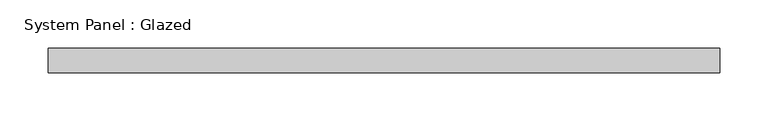
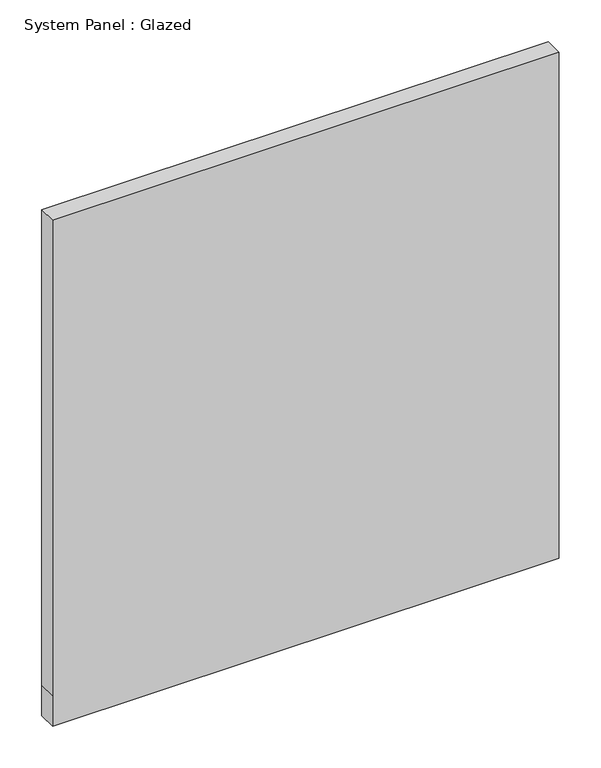
"""IFC4 building model written with IfcOpenShell, lengths in millimetres: plate geometry, System Panel : Glazed."""

from ifc_helpers import new_model, si_unit, frame, origin, place, context, project, spatial, polyline, outline, extrude, source, transform, mapped, element, save


def system_panel_glazed_3a643d3b(model_context):
    return source(origin(), model_context, "Body", "SweptSolid", [
        extrude(outline(polyline([(0.0, -349.25), (0.0, 349.25), (44.45, 349.25), (737.2861093, 349.25), (737.2861093, -349.25), (44.45, -349.25), (0.0, -349.25)])), frame((0.0, 19.05, 0.0), z_axis=(0.0, 1.0, 0.0), x_axis=(0.0, 0.0, 1.0)), (0.0, 0.0, 1.0), 25.4),
    ])


if __name__ == "__main__":
    model = new_model("IFC4")
    model_context = context("Model", 3, world=origin())
    ifc_project = project(units=[si_unit("LENGTHUNIT", "METRE", prefix="MILLI")], contexts=[model_context])
    site = spatial("IfcSite", under=ifc_project)
    building = spatial("IfcBuilding", under=site)
    placement = place(None, origin())
    system_panel_glazed_shape = system_panel_glazed_3a643d3b(model_context)
    element("IfcPlate", 1, ObjectType="System Panel : Glazed", at=placement, inside=building, context=model_context, shape_type="MappedRepresentation", body=[
        mapped(system_panel_glazed_shape, transform((0.0, 0.0, 0.0), x_axis=(1.0, 0.0, 0.0), y_axis=(0.0, 1.0, 0.0), z_axis=(0.0, 0.0, 1.0))),
    ])
    save(model, "model.ifc")

# Revit data of these elements
# Type "System Panel : Glazed"
#   Construction Type Id = "GSP4R"
#   Analytic Construction = "1/8 in Pilkington single glazing"
#   Visual Light Transmittance = 0.9
#   Solar Heat Gain Coefficient = 0.86
#   Heat Transfer Coefficient (U) = 1.18115 BTU/(h·ft²·°F)
#   Define Thermal Properties by = 1
# Element 1 (IfcPlate, "System Panel : Glazed")
#   Materials on its faces: "Glass"
# Materials
#   "Glass": class "Glass", colour RGB 0 128 192, transparency 0.75, Description = "Soda Lime Glass", Cost = 0
